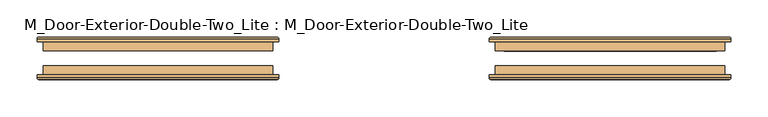
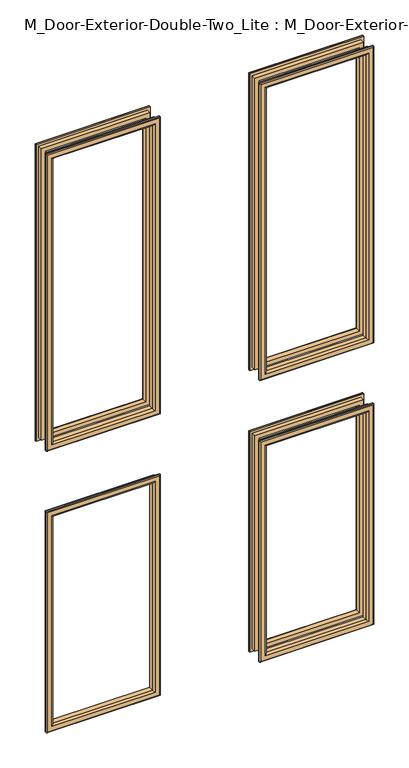
"""IFC4 building model written with IfcOpenShell, lengths in millimetres: door geometry, M_Door-Exterior-Double-Two_Lite : M_Door-Exterior-Double-Two_Lite."""

from ifc_helpers import new_model, si_unit, frame, origin, place, context, project, spatial, ellipse_curve, source, transform, mapped, element, save
from ifc_brep_helpers import plane_surface, cylinder_surface, advanced_brep


def m_door_exterior_double_two_lite_m_door_exterior_double_two_3ba58653(model_context):
    return source(origin(), model_context, "Body", "AdvancedBrep", [
        advanced_brep(
        [(-459.6, 63.15, 1100.0), (-459.6, 50.65, 1100.0), (-459.6, 50.65, 1980.0), (-459.6, 63.15, 1980.0), (-447.6, 49.65, 1112.0), (-447.6, 63.15, 1112.0), (-447.6, 63.15, 1968.0), (-447.6, 49.65, 1968.0), (-452.6, 44.65, 1107.0), (-452.6, 44.65, 1973.0), (-467.6, 46.65, 1092.0), (-465.6, 44.65, 1094.0), (-465.6, 44.65, 1986.0), (-467.6, 46.65, 1988.0), (-467.6, 50.65, 1092.0), (-467.6, 50.65, 1988.0), (-150.0, 50.65, 1980.0), (-150.0, 63.15, 1980.0), (-162.0, 63.15, 1968.0), (-162.0, 49.65, 1968.0), (-157.0, 44.65, 1973.0), (-144.0, 44.65, 1986.0), (-142.0, 46.65, 1988.0), (-142.0, 50.65, 1988.0), (-150.0, 50.65, 1100.0), (-150.0, 63.15, 1100.0), (-162.0, 63.15, 1112.0), (-162.0, 49.65, 1112.0), (-157.0, 44.65, 1107.0), (-144.0, 44.65, 1094.0), (-142.0, 46.65, 1092.0), (-142.0, 50.65, 1092.0)],
        [
            (0, 1),
            (1, 2),
            (2, 3),
            (3, 0),
            (4, 5),
            (5, 6),
            (6, 7),
            (7, 4),
            (8, 4, ellipse_curve(frame((-452.6, 49.65, 1107.0), z_axis=(-0.7071067811865475, 0.0, 0.7071067811865475), x_axis=(-0.7071067811865474, 0.0, -0.7071067811865476)), 7.0710678, 5.0)),
            (7, 9, ellipse_curve(frame((-452.6, 49.65, 1973.0), z_axis=(-0.7071067811865475, 0.0, -0.7071067811865475), x_axis=(0.7071067811865474, 0.0, -0.7071067811865476)), 7.0710678, 5.0)),
            (9, 8),
            (10, 11, ellipse_curve(frame((-465.6, 46.65, 1094.0), z_axis=(-0.7071067811865475, 0.0, 0.7071067811865475), x_axis=(-0.7071067811865474, 0.0, -0.7071067811865476)), 2.8284271, 2.0)),
            (11, 12),
            (12, 13, ellipse_curve(frame((-465.6, 46.65, 1986.0), z_axis=(-0.7071067811865475, 0.0, -0.7071067811865475), x_axis=(0.7071067811865474, 0.0, -0.7071067811865476)), 2.8284271, 2.0)),
            (13, 10),
            (14, 10),
            (13, 15),
            (15, 14),
            (2, 16),
            (16, 17),
            (17, 3),
            (6, 18),
            (18, 19),
            (19, 7),
            (19, 20, ellipse_curve(frame((-157.0, 49.65, 1973.0), z_axis=(-0.7071067811865475, 0.0, 0.7071067811865475), x_axis=(-0.7071067811865476, 0.0, -0.7071067811865474)), 7.0710678, 5.0)),
            (20, 9),
            (12, 21),
            (21, 22, ellipse_curve(frame((-144.0, 46.65, 1986.0), z_axis=(-0.7071067811865475, 0.0, 0.7071067811865475), x_axis=(-0.7071067811865476, 0.0, -0.7071067811865474)), 2.8284271, 2.0)),
            (22, 13),
            (22, 23),
            (23, 15),
            (16, 24),
            (24, 25),
            (25, 17),
            (18, 26),
            (26, 27),
            (27, 19),
            (27, 28, ellipse_curve(frame((-157.0, 49.65, 1107.0), z_axis=(0.7071067811865475, 0.0, 0.7071067811865475), x_axis=(-0.7071067811865474, 0.0, 0.7071067811865476)), 7.0710678, 5.0)),
            (28, 20),
            (21, 29),
            (29, 30, ellipse_curve(frame((-144.0, 46.65, 1094.0), z_axis=(0.7071067811865475, 0.0, 0.7071067811865475), x_axis=(-0.7071067811865474, 0.0, 0.7071067811865476)), 2.8284271, 2.0)),
            (30, 22),
            (30, 31),
            (31, 23),
            (31, 14),
            (1, 24),
            (0, 25),
            (5, 26),
            (4, 27),
            (8, 28),
            (11, 29),
            (10, 30),
        ],
        [
            plane_surface(frame((-459.6, 50.65, 1100.0), z_axis=(-1.0, 0.0, 0.0), x_axis=(0.0, 0.0, 1.0))),
            plane_surface(frame((-447.6, 63.15, 1112.0), z_axis=(1.0, 0.0, 0.0), x_axis=(0.0, 0.0, 1.0))),
            cylinder_surface(frame((-452.6, 49.65, 1100.0), z_axis=(0.0, 0.0, -1.0), x_axis=(-1.0, 0.0, 0.0)), 5.0),
            cylinder_surface(frame((-465.6, 46.65, 1100.0), z_axis=(0.0, 0.0, -1.0), x_axis=(-1.0, 0.0, 0.0)), 2.0),
            plane_surface(frame((-467.6, 46.65, 1092.0), z_axis=(-1.0, 0.0, 0.0), x_axis=(0.0, 0.0, 1.0))),
            plane_surface(frame((-459.6, 50.65, 1980.0), z_axis=(0.0, 0.0, 1.0), x_axis=(1.0, 0.0, 0.0))),
            plane_surface(frame((-447.6, 63.15, 1968.0), z_axis=(0.0, 0.0, -1.0), x_axis=(1.0, 0.0, 0.0))),
            cylinder_surface(frame((-459.6, 49.65, 1973.0), z_axis=(-1.0, 0.0, 0.0), x_axis=(0.0, 0.0, 1.0)), 5.0),
            cylinder_surface(frame((-459.6, 46.65, 1986.0), z_axis=(-1.0, 0.0, 0.0), x_axis=(0.0, 0.0, 1.0)), 2.0),
            plane_surface(frame((-467.6, 46.65, 1988.0), z_axis=(0.0, 0.0, 1.0), x_axis=(1.0, 0.0, 0.0))),
            plane_surface(frame((-150.0, 50.65, 1980.0), z_axis=(1.0, 0.0, 0.0), x_axis=(0.0, 0.0, -1.0))),
            plane_surface(frame((-162.0, 63.15, 1968.0), z_axis=(-1.0, 0.0, 0.0), x_axis=(0.0, 0.0, -1.0))),
            cylinder_surface(frame((-157.0, 49.65, 1980.0), z_axis=(0.0, 0.0, 1.0), x_axis=(1.0, 0.0, 0.0)), 5.0),
            cylinder_surface(frame((-144.0, 46.65, 1980.0), z_axis=(0.0, 0.0, 1.0), x_axis=(1.0, 0.0, 0.0)), 2.0),
            plane_surface(frame((-142.0, 46.65, 1988.0), z_axis=(1.0, 0.0, 0.0), x_axis=(0.0, 0.0, -1.0))),
            plane_surface(frame((-142.0, 50.65, 1092.0), z_axis=(0.0, 1.0, 0.0), x_axis=(-1.0, 0.0, 0.0))),
            plane_surface(frame((-150.0, 50.65, 1100.0), z_axis=(0.0, 0.0, -1.0), x_axis=(-1.0, 0.0, 0.0))),
            plane_surface(frame((-150.0, 63.15, 1100.0), z_axis=(0.0, 1.0, 0.0), x_axis=(-1.0, 0.0, 0.0))),
            plane_surface(frame((-162.0, 63.15, 1112.0), z_axis=(0.0, 0.0, 1.0), x_axis=(-1.0, 0.0, 0.0))),
            cylinder_surface(frame((-150.0, 49.65, 1107.0), z_axis=(1.0, 0.0, 0.0), x_axis=(0.0, 0.0, -1.0)), 5.0),
            plane_surface(frame((-157.0, 44.65, 1107.0), z_axis=(0.0, -1.0, 0.0), x_axis=(-1.0, 0.0, 0.0))),
            cylinder_surface(frame((-150.0, 46.65, 1094.0), z_axis=(1.0, 0.0, 0.0), x_axis=(0.0, 0.0, -1.0)), 2.0),
            plane_surface(frame((-142.0, 46.65, 1092.0), z_axis=(0.0, 0.0, -1.0), x_axis=(-1.0, 0.0, 0.0))),
        ],
        [
            (0, [[1, 2, 3, 4]]),
            (1, [[5, 6, 7, 8]]),
            (2, [[9, -8, 10, 11]]),
            (3, [[12, 13, 14, 15]]),
            (4, [[16, -15, 17, 18]]),
            (5, [[-3, 19, 20, 21]]),
            (6, [[-7, 22, 23, 24]]),
            (7, [[-10, -24, 25, 26]]),
            (8, [[-14, 27, 28, 29]]),
            (9, [[-17, -29, 30, 31]]),
            (10, [[-20, 32, 33, 34]]),
            (11, [[-23, 35, 36, 37]]),
            (12, [[-25, -37, 38, 39]]),
            (13, [[-28, 40, 41, 42]]),
            (14, [[-30, -42, 43, 44]]),
            (15, [[-31, -44, 45, -18], [46, -32, -19, -2]]),
            (16, [[-33, -46, -1, 47]]),
            (17, [[-21, -34, -47, -4], [48, -35, -22, -6]]),
            (18, [[-36, -48, -5, 49]]),
            (19, [[-38, -49, -9, 50]]),
            (20, [[51, -40, -27, -13], [-26, -39, -50, -11]]),
            (21, [[-41, -51, -12, 52]]),
            (22, [[-43, -52, -16, -45]]),
        ],
    ),
        advanced_brep(
        [(150.0, 63.15, 1100.0), (150.0, 50.65, 1100.0), (150.0, 50.65, 1980.0), (150.0, 63.15, 1980.0), (162.0, 49.65, 1112.0), (162.0, 63.15, 1112.0), (162.0, 63.15, 1968.0), (162.0, 49.65, 1968.0), (157.0, 44.65, 1107.0), (157.0, 44.65, 1973.0), (142.0, 46.65, 1092.0), (144.0, 44.65, 1094.0), (144.0, 44.65, 1986.0), (142.0, 46.65, 1988.0), (142.0, 50.65, 1092.0), (142.0, 50.65, 1988.0), (459.6, 50.65, 1980.0), (459.6, 63.15, 1980.0), (447.6, 63.15, 1968.0), (447.6, 49.65, 1968.0), (452.6, 44.65, 1973.0), (465.6, 44.65, 1986.0), (467.6, 46.65, 1988.0), (467.6, 50.65, 1988.0), (459.6, 50.65, 1100.0), (459.6, 63.15, 1100.0), (447.6, 63.15, 1112.0), (447.6, 49.65, 1112.0), (452.6, 44.65, 1107.0), (465.6, 44.65, 1094.0), (467.6, 46.65, 1092.0), (467.6, 50.65, 1092.0)],
        [
            (0, 1),
            (1, 2),
            (2, 3),
            (3, 0),
            (4, 5),
            (5, 6),
            (6, 7),
            (7, 4),
            (8, 4, ellipse_curve(frame((157.0, 49.65, 1107.0), z_axis=(-0.7071067811865475, 0.0, 0.7071067811865475), x_axis=(-0.7071067811865474, 0.0, -0.7071067811865476)), 7.0710678, 5.0)),
            (7, 9, ellipse_curve(frame((157.0, 49.65, 1973.0), z_axis=(-0.7071067811865475, 0.0, -0.7071067811865475), x_axis=(0.7071067811865474, 0.0, -0.7071067811865476)), 7.0710678, 5.0)),
            (9, 8),
            (10, 11, ellipse_curve(frame((144.0, 46.65, 1094.0), z_axis=(-0.7071067811865475, 0.0, 0.7071067811865475), x_axis=(-0.7071067811865474, 0.0, -0.7071067811865476)), 2.8284271, 2.0)),
            (11, 12),
            (12, 13, ellipse_curve(frame((144.0, 46.65, 1986.0), z_axis=(-0.7071067811865475, 0.0, -0.7071067811865475), x_axis=(0.7071067811865474, 0.0, -0.7071067811865476)), 2.8284271, 2.0)),
            (13, 10),
            (14, 10),
            (13, 15),
            (15, 14),
            (2, 16),
            (16, 17),
            (17, 3),
            (6, 18),
            (18, 19),
            (19, 7),
            (19, 20, ellipse_curve(frame((452.6, 49.65, 1973.0), z_axis=(-0.7071067811865475, 0.0, 0.7071067811865475), x_axis=(-0.7071067811865476, 0.0, -0.7071067811865474)), 7.0710678, 5.0)),
            (20, 9),
            (12, 21),
            (21, 22, ellipse_curve(frame((465.6, 46.65, 1986.0), z_axis=(-0.7071067811865475, 0.0, 0.7071067811865475), x_axis=(-0.7071067811865476, 0.0, -0.7071067811865474)), 2.8284271, 2.0)),
            (22, 13),
            (22, 23),
            (23, 15),
            (16, 24),
            (24, 25),
            (25, 17),
            (18, 26),
            (26, 27),
            (27, 19),
            (27, 28, ellipse_curve(frame((452.6, 49.65, 1107.0), z_axis=(0.7071067811865475, 0.0, 0.7071067811865475), x_axis=(-0.7071067811865474, 0.0, 0.7071067811865476)), 7.0710678, 5.0)),
            (28, 20),
            (21, 29),
            (29, 30, ellipse_curve(frame((465.6, 46.65, 1094.0), z_axis=(0.7071067811865475, 0.0, 0.7071067811865475), x_axis=(-0.7071067811865474, 0.0, 0.7071067811865476)), 2.8284271, 2.0)),
            (30, 22),
            (30, 31),
            (31, 23),
            (31, 14),
            (1, 24),
            (0, 25),
            (5, 26),
            (4, 27),
            (8, 28),
            (11, 29),
            (10, 30),
        ],
        [
            plane_surface(frame((150.0, 50.65, 1100.0), z_axis=(-1.0, 0.0, 0.0), x_axis=(0.0, 0.0, 1.0))),
            plane_surface(frame((162.0, 63.15, 1112.0), z_axis=(1.0, 0.0, 0.0), x_axis=(0.0, 0.0, 1.0))),
            cylinder_surface(frame((157.0, 49.65, 1100.0), z_axis=(0.0, 0.0, -1.0), x_axis=(-1.0, 0.0, 0.0)), 5.0),
            cylinder_surface(frame((144.0, 46.65, 1100.0), z_axis=(0.0, 0.0, -1.0), x_axis=(-1.0, 0.0, 0.0)), 2.0),
            plane_surface(frame((142.0, 46.65, 1092.0), z_axis=(-1.0, 0.0, 0.0), x_axis=(0.0, 0.0, 1.0))),
            plane_surface(frame((150.0, 50.65, 1980.0), z_axis=(0.0, 0.0, 1.0), x_axis=(1.0, 0.0, 0.0))),
            plane_surface(frame((162.0, 63.15, 1968.0), z_axis=(0.0, 0.0, -1.0), x_axis=(1.0, 0.0, 0.0))),
            cylinder_surface(frame((150.0, 49.65, 1973.0), z_axis=(-1.0, 0.0, 0.0), x_axis=(0.0, 0.0, 1.0)), 5.0),
            cylinder_surface(frame((150.0, 46.65, 1986.0), z_axis=(-1.0, 0.0, 0.0), x_axis=(0.0, 0.0, 1.0)), 2.0),
            plane_surface(frame((142.0, 46.65, 1988.0), z_axis=(0.0, 0.0, 1.0), x_axis=(1.0, 0.0, 0.0))),
            plane_surface(frame((459.6, 50.65, 1980.0), z_axis=(1.0, 0.0, 0.0), x_axis=(0.0, 0.0, -1.0))),
            plane_surface(frame((447.6, 63.15, 1968.0), z_axis=(-1.0, 0.0, 0.0), x_axis=(0.0, 0.0, -1.0))),
            cylinder_surface(frame((452.6, 49.65, 1980.0), z_axis=(0.0, 0.0, 1.0), x_axis=(1.0, 0.0, 0.0)), 5.0),
            cylinder_surface(frame((465.6, 46.65, 1980.0), z_axis=(0.0, 0.0, 1.0), x_axis=(1.0, 0.0, 0.0)), 2.0),
            plane_surface(frame((467.6, 46.65, 1988.0), z_axis=(1.0, 0.0, 0.0), x_axis=(0.0, 0.0, -1.0))),
            plane_surface(frame((467.6, 50.65, 1092.0), z_axis=(0.0, 1.0, 0.0), x_axis=(-1.0, 0.0, 0.0))),
            plane_surface(frame((459.6, 50.65, 1100.0), z_axis=(0.0, 0.0, -1.0), x_axis=(-1.0, 0.0, 0.0))),
            plane_surface(frame((459.6, 63.15, 1100.0), z_axis=(0.0, 1.0, 0.0), x_axis=(-1.0, 0.0, 0.0))),
            plane_surface(frame((447.6, 63.15, 1112.0), z_axis=(0.0, 0.0, 1.0), x_axis=(-1.0, 0.0, 0.0))),
            cylinder_surface(frame((459.6, 49.65, 1107.0), z_axis=(1.0, 0.0, 0.0), x_axis=(0.0, 0.0, -1.0)), 5.0),
            plane_surface(frame((452.6, 44.65, 1107.0), z_axis=(0.0, -1.0, 0.0), x_axis=(-1.0, 0.0, 0.0))),
            cylinder_surface(frame((459.6, 46.65, 1094.0), z_axis=(1.0, 0.0, 0.0), x_axis=(0.0, 0.0, -1.0)), 2.0),
            plane_surface(frame((467.6, 46.65, 1092.0), z_axis=(0.0, 0.0, -1.0), x_axis=(-1.0, 0.0, 0.0))),
        ],
        [
            (0, [[1, 2, 3, 4]]),
            (1, [[5, 6, 7, 8]]),
            (2, [[9, -8, 10, 11]]),
            (3, [[12, 13, 14, 15]]),
            (4, [[16, -15, 17, 18]]),
            (5, [[-3, 19, 20, 21]]),
            (6, [[-7, 22, 23, 24]]),
            (7, [[-10, -24, 25, 26]]),
            (8, [[-14, 27, 28, 29]]),
            (9, [[-17, -29, 30, 31]]),
            (10, [[-20, 32, 33, 34]]),
            (11, [[-23, 35, 36, 37]]),
            (12, [[-25, -37, 38, 39]]),
            (13, [[-28, 40, 41, 42]]),
            (14, [[-30, -42, 43, 44]]),
            (15, [[-31, -44, 45, -18], [46, -32, -19, -2]]),
            (16, [[-33, -46, -1, 47]]),
            (17, [[-21, -34, -47, -4], [48, -35, -22, -6]]),
            (18, [[-36, -48, -5, 49]]),
            (19, [[-38, -49, -9, 50]]),
            (20, [[51, -40, -27, -13], [-26, -39, -50, -11]]),
            (21, [[-41, -51, -12, 52]]),
            (22, [[-43, -52, -16, -45]]),
        ],
    ),
        advanced_brep(
        [(150.0, 63.15, 250.0), (150.0, 50.65, 250.0), (150.0, 50.65, 900.0), (150.0, 63.15, 900.0), (162.0, 49.65, 262.0), (162.0, 63.15, 262.0), (162.0, 63.15, 888.0), (162.0, 49.65, 888.0), (157.0, 44.65, 257.0), (157.0, 44.65, 893.0), (142.0, 46.65, 242.0), (144.0, 44.65, 244.0), (144.0, 44.65, 906.0), (142.0, 46.65, 908.0), (142.0, 50.65, 242.0), (142.0, 50.65, 908.0), (459.6, 50.65, 900.0), (459.6, 63.15, 900.0), (447.6, 63.15, 888.0), (447.6, 49.65, 888.0), (452.6, 44.65, 893.0), (465.6, 44.65, 906.0), (467.6, 46.65, 908.0), (467.6, 50.65, 908.0), (459.6, 50.65, 250.0), (459.6, 63.15, 250.0), (447.6, 63.15, 262.0), (447.6, 49.65, 262.0), (452.6, 44.65, 257.0), (465.6, 44.65, 244.0), (467.6, 46.65, 242.0), (467.6, 50.65, 242.0)],
        [
            (0, 1),
            (1, 2),
            (2, 3),
            (3, 0),
            (4, 5),
            (5, 6),
            (6, 7),
            (7, 4),
            (8, 4, ellipse_curve(frame((157.0, 49.65, 257.0), z_axis=(-0.7071067811865475, 0.0, 0.7071067811865475), x_axis=(-0.7071067811865474, 0.0, -0.7071067811865476)), 7.0710678, 5.0)),
            (7, 9, ellipse_curve(frame((157.0, 49.65, 893.0), z_axis=(-0.7071067811865475, 0.0, -0.7071067811865475), x_axis=(0.7071067811865474, 0.0, -0.7071067811865476)), 7.0710678, 5.0)),
            (9, 8),
            (10, 11, ellipse_curve(frame((144.0, 46.65, 244.0), z_axis=(-0.7071067811865475, 0.0, 0.7071067811865475), x_axis=(-0.7071067811865474, 0.0, -0.7071067811865476)), 2.8284271, 2.0)),
            (11, 12),
            (12, 13, ellipse_curve(frame((144.0, 46.65, 906.0), z_axis=(-0.7071067811865475, 0.0, -0.7071067811865475), x_axis=(0.7071067811865474, 0.0, -0.7071067811865476)), 2.8284271, 2.0)),
            (13, 10),
            (14, 10),
            (13, 15),
            (15, 14),
            (2, 16),
            (16, 17),
            (17, 3),
            (6, 18),
            (18, 19),
            (19, 7),
            (19, 20, ellipse_curve(frame((452.6, 49.65, 893.0), z_axis=(-0.7071067811865475, 0.0, 0.7071067811865475), x_axis=(-0.7071067811865476, 0.0, -0.7071067811865474)), 7.0710678, 5.0)),
            (20, 9),
            (12, 21),
            (21, 22, ellipse_curve(frame((465.6, 46.65, 906.0), z_axis=(-0.7071067811865475, 0.0, 0.7071067811865475), x_axis=(-0.7071067811865476, 0.0, -0.7071067811865474)), 2.8284271, 2.0)),
            (22, 13),
            (22, 23),
            (23, 15),
            (16, 24),
            (24, 25),
            (25, 17),
            (18, 26),
            (26, 27),
            (27, 19),
            (27, 28, ellipse_curve(frame((452.6, 49.65, 257.0), z_axis=(0.7071067811865475, 0.0, 0.7071067811865475), x_axis=(-0.7071067811865474, 0.0, 0.7071067811865476)), 7.0710678, 5.0)),
            (28, 20),
            (21, 29),
            (29, 30, ellipse_curve(frame((465.6, 46.65, 244.0), z_axis=(0.7071067811865475, 0.0, 0.7071067811865475), x_axis=(-0.7071067811865474, 0.0, 0.7071067811865476)), 2.8284271, 2.0)),
            (30, 22),
            (30, 31),
            (31, 23),
            (31, 14),
            (1, 24),
            (0, 25),
            (5, 26),
            (4, 27),
            (8, 28),
            (11, 29),
            (10, 30),
        ],
        [
            plane_surface(frame((150.0, 50.65, 250.0), z_axis=(-1.0, 0.0, 0.0), x_axis=(0.0, 0.0, 1.0))),
            plane_surface(frame((162.0, 63.15, 262.0), z_axis=(1.0, 0.0, 0.0), x_axis=(0.0, 0.0, 1.0))),
            cylinder_surface(frame((157.0, 49.65, 250.0), z_axis=(0.0, 0.0, -1.0), x_axis=(-1.0, 0.0, 0.0)), 5.0),
            cylinder_surface(frame((144.0, 46.65, 250.0), z_axis=(0.0, 0.0, -1.0), x_axis=(-1.0, 0.0, 0.0)), 2.0),
            plane_surface(frame((142.0, 46.65, 242.0), z_axis=(-1.0, 0.0, 0.0), x_axis=(0.0, 0.0, 1.0))),
            plane_surface(frame((150.0, 50.65, 900.0), z_axis=(0.0, 0.0, 1.0), x_axis=(1.0, 0.0, 0.0))),
            plane_surface(frame((162.0, 63.15, 888.0), z_axis=(0.0, 0.0, -1.0), x_axis=(1.0, 0.0, 0.0))),
            cylinder_surface(frame((150.0, 49.65, 893.0), z_axis=(-1.0, 0.0, 0.0), x_axis=(0.0, 0.0, 1.0)), 5.0),
            cylinder_surface(frame((150.0, 46.65, 906.0), z_axis=(-1.0, 0.0, 0.0), x_axis=(0.0, 0.0, 1.0)), 2.0),
            plane_surface(frame((142.0, 46.65, 908.0), z_axis=(0.0, 0.0, 1.0), x_axis=(1.0, 0.0, 0.0))),
            plane_surface(frame((459.6, 50.65, 900.0), z_axis=(1.0, 0.0, 0.0), x_axis=(0.0, 0.0, -1.0))),
            plane_surface(frame((447.6, 63.15, 888.0), z_axis=(-1.0, 0.0, 0.0), x_axis=(0.0, 0.0, -1.0))),
            cylinder_surface(frame((452.6, 49.65, 900.0), z_axis=(0.0, 0.0, 1.0), x_axis=(1.0, 0.0, 0.0)), 5.0),
            cylinder_surface(frame((465.6, 46.65, 900.0), z_axis=(0.0, 0.0, 1.0), x_axis=(1.0, 0.0, 0.0)), 2.0),
            plane_surface(frame((467.6, 46.65, 908.0), z_axis=(1.0, 0.0, 0.0), x_axis=(0.0, 0.0, -1.0))),
            plane_surface(frame((467.6, 50.65, 242.0), z_axis=(0.0, 1.0, 0.0), x_axis=(-1.0, 0.0, 0.0))),
            plane_surface(frame((459.6, 50.65, 250.0), z_axis=(0.0, 0.0, -1.0), x_axis=(-1.0, 0.0, 0.0))),
            plane_surface(frame((459.6, 63.15, 250.0), z_axis=(0.0, 1.0, 0.0), x_axis=(-1.0, 0.0, 0.0))),
            plane_surface(frame((447.6, 63.15, 262.0), z_axis=(0.0, 0.0, 1.0), x_axis=(-1.0, 0.0, 0.0))),
            cylinder_surface(frame((459.6, 49.65, 257.0), z_axis=(1.0, 0.0, 0.0), x_axis=(0.0, 0.0, -1.0)), 5.0),
            plane_surface(frame((452.6, 44.65, 257.0), z_axis=(0.0, -1.0, 0.0), x_axis=(-1.0, 0.0, 0.0))),
            cylinder_surface(frame((459.6, 46.65, 244.0), z_axis=(1.0, 0.0, 0.0), x_axis=(0.0, 0.0, -1.0)), 2.0),
            plane_surface(frame((467.6, 46.65, 242.0), z_axis=(0.0, 0.0, -1.0), x_axis=(-1.0, 0.0, 0.0))),
        ],
        [
            (0, [[1, 2, 3, 4]]),
            (1, [[5, 6, 7, 8]]),
            (2, [[9, -8, 10, 11]]),
            (3, [[12, 13, 14, 15]]),
            (4, [[16, -15, 17, 18]]),
            (5, [[-3, 19, 20, 21]]),
            (6, [[-7, 22, 23, 24]]),
            (7, [[-10, -24, 25, 26]]),
            (8, [[-14, 27, 28, 29]]),
            (9, [[-17, -29, 30, 31]]),
            (10, [[-20, 32, 33, 34]]),
            (11, [[-23, 35, 36, 37]]),
            (12, [[-25, -37, 38, 39]]),
            (13, [[-28, 40, 41, 42]]),
            (14, [[-30, -42, 43, 44]]),
            (15, [[-31, -44, 45, -18], [46, -32, -19, -2]]),
            (16, [[-33, -46, -1, 47]]),
            (17, [[-21, -34, -47, -4], [48, -35, -22, -6]]),
            (18, [[-36, -48, -5, 49]]),
            (19, [[-38, -49, -9, 50]]),
            (20, [[51, -40, -27, -13], [-26, -39, -50, -11]]),
            (21, [[-41, -51, -12, 52]]),
            (22, [[-43, -52, -16, -45]]),
        ],
    ),
        advanced_brep(
        [(-459.6, 63.15, 250.0), (-459.6, 50.65, 250.0), (-459.6, 50.65, 900.0), (-459.6, 63.15, 900.0), (-447.6, 49.65, 262.0), (-447.6, 63.15, 262.0), (-447.6, 63.15, 888.0), (-447.6, 49.65, 888.0), (-452.6, 44.65, 257.0), (-452.6, 44.65, 893.0), (-467.6, 46.65, 242.0), (-465.6, 44.65, 244.0), (-465.6, 44.65, 906.0), (-467.6, 46.65, 908.0), (-467.6, 50.65, 242.0), (-467.6, 50.65, 908.0), (-150.0, 50.65, 900.0), (-150.0, 63.15, 900.0), (-162.0, 63.15, 888.0), (-162.0, 49.65, 888.0), (-157.0, 44.65, 893.0), (-144.0, 44.65, 906.0), (-142.0, 46.65, 908.0), (-142.0, 50.65, 908.0), (-150.0, 50.65, 250.0), (-150.0, 63.15, 250.0), (-162.0, 63.15, 262.0), (-162.0, 49.65, 262.0), (-157.0, 44.65, 257.0), (-144.0, 44.65, 244.0), (-142.0, 46.65, 242.0), (-142.0, 50.65, 242.0)],
        [
            (0, 1),
            (1, 2),
            (2, 3),
            (3, 0),
            (4, 5),
            (5, 6),
            (6, 7),
            (7, 4),
            (8, 4, ellipse_curve(frame((-452.6, 49.65, 257.0), z_axis=(-0.7071067811865475, 0.0, 0.7071067811865475), x_axis=(-0.7071067811865474, 0.0, -0.7071067811865476)), 7.0710678, 5.0)),
            (7, 9, ellipse_curve(frame((-452.6, 49.65, 893.0), z_axis=(-0.7071067811865475, 0.0, -0.7071067811865475), x_axis=(0.7071067811865474, 0.0, -0.7071067811865476)), 7.0710678, 5.0)),
            (9, 8),
            (10, 11, ellipse_curve(frame((-465.6, 46.65, 244.0), z_axis=(-0.7071067811865475, 0.0, 0.7071067811865475), x_axis=(-0.7071067811865474, 0.0, -0.7071067811865476)), 2.8284271, 2.0)),
            (11, 12),
            (12, 13, ellipse_curve(frame((-465.6, 46.65, 906.0), z_axis=(-0.7071067811865475, 0.0, -0.7071067811865475), x_axis=(0.7071067811865474, 0.0, -0.7071067811865476)), 2.8284271, 2.0)),
            (13, 10),
            (14, 10),
            (13, 15),
            (15, 14),
            (2, 16),
            (16, 17),
            (17, 3),
            (6, 18),
            (18, 19),
            (19, 7),
            (19, 20, ellipse_curve(frame((-157.0, 49.65, 893.0), z_axis=(-0.7071067811865475, 0.0, 0.7071067811865475), x_axis=(-0.7071067811865476, 0.0, -0.7071067811865474)), 7.0710678, 5.0)),
            (20, 9),
            (12, 21),
            (21, 22, ellipse_curve(frame((-144.0, 46.65, 906.0), z_axis=(-0.7071067811865475, 0.0, 0.7071067811865475), x_axis=(-0.7071067811865476, 0.0, -0.7071067811865474)), 2.8284271, 2.0)),
            (22, 13),
            (22, 23),
            (23, 15),
            (16, 24),
            (24, 25),
            (25, 17),
            (18, 26),
            (26, 27),
            (27, 19),
            (27, 28, ellipse_curve(frame((-157.0, 49.65, 257.0), z_axis=(0.7071067811865475, 0.0, 0.7071067811865475), x_axis=(-0.7071067811865474, 0.0, 0.7071067811865476)), 7.0710678, 5.0)),
            (28, 20),
            (21, 29),
            (29, 30, ellipse_curve(frame((-144.0, 46.65, 244.0), z_axis=(0.7071067811865475, 0.0, 0.7071067811865475), x_axis=(-0.7071067811865474, 0.0, 0.7071067811865476)), 2.8284271, 2.0)),
            (30, 22),
            (30, 31),
            (31, 23),
            (31, 14),
            (1, 24),
            (0, 25),
            (5, 26),
            (4, 27),
            (8, 28),
            (11, 29),
            (10, 30),
        ],
        [
            plane_surface(frame((-459.6, 50.65, 250.0), z_axis=(-1.0, 0.0, 0.0), x_axis=(0.0, 0.0, 1.0))),
            plane_surface(frame((-447.6, 63.15, 262.0), z_axis=(1.0, 0.0, 0.0), x_axis=(0.0, 0.0, 1.0))),
            cylinder_surface(frame((-452.6, 49.65, 250.0), z_axis=(0.0, 0.0, -1.0), x_axis=(-1.0, 0.0, 0.0)), 5.0),
            cylinder_surface(frame((-465.6, 46.65, 250.0), z_axis=(0.0, 0.0, -1.0), x_axis=(-1.0, 0.0, 0.0)), 2.0),
            plane_surface(frame((-467.6, 46.65, 242.0), z_axis=(-1.0, 0.0, 0.0), x_axis=(0.0, 0.0, 1.0))),
            plane_surface(frame((-459.6, 50.65, 900.0), z_axis=(0.0, 0.0, 1.0), x_axis=(1.0, 0.0, 0.0))),
            plane_surface(frame((-447.6, 63.15, 888.0), z_axis=(0.0, 0.0, -1.0), x_axis=(1.0, 0.0, 0.0))),
            cylinder_surface(frame((-459.6, 49.65, 893.0), z_axis=(-1.0, 0.0, 0.0), x_axis=(0.0, 0.0, 1.0)), 5.0),
            cylinder_surface(frame((-459.6, 46.65, 906.0), z_axis=(-1.0, 0.0, 0.0), x_axis=(0.0, 0.0, 1.0)), 2.0),
            plane_surface(frame((-467.6, 46.65, 908.0), z_axis=(0.0, 0.0, 1.0), x_axis=(1.0, 0.0, 0.0))),
            plane_surface(frame((-150.0, 50.65, 900.0), z_axis=(1.0, 0.0, 0.0), x_axis=(0.0, 0.0, -1.0))),
            plane_surface(frame((-162.0, 63.15, 888.0), z_axis=(-1.0, 0.0, 0.0), x_axis=(0.0, 0.0, -1.0))),
            cylinder_surface(frame((-157.0, 49.65, 900.0), z_axis=(0.0, 0.0, 1.0), x_axis=(1.0, 0.0, 0.0)), 5.0),
            cylinder_surface(frame((-144.0, 46.65, 900.0), z_axis=(0.0, 0.0, 1.0), x_axis=(1.0, 0.0, 0.0)), 2.0),
            plane_surface(frame((-142.0, 46.65, 908.0), z_axis=(1.0, 0.0, 0.0), x_axis=(0.0, 0.0, -1.0))),
            plane_surface(frame((-142.0, 50.65, 242.0), z_axis=(0.0, 1.0, 0.0), x_axis=(-1.0, 0.0, 0.0))),
            plane_surface(frame((-150.0, 50.65, 250.0), z_axis=(0.0, 0.0, -1.0), x_axis=(-1.0, 0.0, 0.0))),
            plane_surface(frame((-150.0, 63.15, 250.0), z_axis=(0.0, 1.0, 0.0), x_axis=(-1.0, 0.0, 0.0))),
            plane_surface(frame((-162.0, 63.15, 262.0), z_axis=(0.0, 0.0, 1.0), x_axis=(-1.0, 0.0, 0.0))),
            cylinder_surface(frame((-150.0, 49.65, 257.0), z_axis=(1.0, 0.0, 0.0), x_axis=(0.0, 0.0, -1.0)), 5.0),
            plane_surface(frame((-157.0, 44.65, 257.0), z_axis=(0.0, -1.0, 0.0), x_axis=(-1.0, 0.0, 0.0))),
            cylinder_surface(frame((-150.0, 46.65, 244.0), z_axis=(1.0, 0.0, 0.0), x_axis=(0.0, 0.0, -1.0)), 2.0),
            plane_surface(frame((-142.0, 46.65, 242.0), z_axis=(0.0, 0.0, -1.0), x_axis=(-1.0, 0.0, 0.0))),
        ],
        [
            (0, [[1, 2, 3, 4]]),
            (1, [[5, 6, 7, 8]]),
            (2, [[9, -8, 10, 11]]),
            (3, [[12, 13, 14, 15]]),
            (4, [[16, -15, 17, 18]]),
            (5, [[-3, 19, 20, 21]]),
            (6, [[-7, 22, 23, 24]]),
            (7, [[-10, -24, 25, 26]]),
            (8, [[-14, 27, 28, 29]]),
            (9, [[-17, -29, 30, 31]]),
            (10, [[-20, 32, 33, 34]]),
            (11, [[-23, 35, 36, 37]]),
            (12, [[-25, -37, 38, 39]]),
            (13, [[-28, 40, 41, 42]]),
            (14, [[-30, -42, 43, 44]]),
            (15, [[-31, -44, 45, -18], [46, -32, -19, -2]]),
            (16, [[-33, -46, -1, 47]]),
            (17, [[-21, -34, -47, -4], [48, -35, -22, -6]]),
            (18, [[-36, -48, -5, 49]]),
            (19, [[-38, -49, -9, 50]]),
            (20, [[51, -40, -27, -13], [-26, -39, -50, -11]]),
            (21, [[-41, -51, -12, 52]]),
            (22, [[-43, -52, -16, -45]]),
        ],
    ),
        advanced_brep(
        [(-459.6, 83.15, 1980.0), (-459.6, 95.65, 1980.0), (-459.6, 95.65, 1100.0), (-459.6, 83.15, 1100.0), (-447.6, 96.65, 1968.0), (-447.6, 83.15, 1968.0), (-447.6, 83.15, 1112.0), (-447.6, 96.65, 1112.0), (-452.6, 101.65, 1973.0), (-452.6, 101.65, 1107.0), (-467.6, 99.65, 1988.0), (-465.6, 101.65, 1986.0), (-465.6, 101.65, 1094.0), (-467.6, 99.65, 1092.0), (-467.6, 95.65, 1988.0), (-467.6, 95.65, 1092.0), (-150.0, 95.65, 1100.0), (-150.0, 83.15, 1100.0), (-162.0, 83.15, 1112.0), (-162.0, 96.65, 1112.0), (-157.0, 101.65, 1107.0), (-144.0, 101.65, 1094.0), (-142.0, 99.65, 1092.0), (-142.0, 95.65, 1092.0), (-150.0, 95.65, 1980.0), (-150.0, 83.15, 1980.0), (-162.0, 83.15, 1968.0), (-162.0, 96.65, 1968.0), (-157.0, 101.65, 1973.0), (-144.0, 101.65, 1986.0), (-142.0, 99.65, 1988.0), (-142.0, 95.65, 1988.0)],
        [
            (0, 1),
            (1, 2),
            (2, 3),
            (3, 0),
            (4, 5),
            (5, 6),
            (6, 7),
            (7, 4),
            (8, 4, ellipse_curve(frame((-452.6, 96.65, 1973.0), z_axis=(-0.7071067811865475, 0.0, -0.7071067811865475), x_axis=(-0.7071067811865474, 0.0, 0.7071067811865476)), 7.0710678, 5.0)),
            (7, 9, ellipse_curve(frame((-452.6, 96.65, 1107.0), z_axis=(-0.7071067811865475, 0.0, 0.7071067811865475), x_axis=(0.7071067811865474, 0.0, 0.7071067811865476)), 7.0710678, 5.0)),
            (9, 8),
            (10, 11, ellipse_curve(frame((-465.6, 99.65, 1986.0), z_axis=(-0.7071067811865475, 0.0, -0.7071067811865475), x_axis=(-0.7071067811865474, 0.0, 0.7071067811865476)), 2.8284271, 2.0)),
            (11, 12),
            (12, 13, ellipse_curve(frame((-465.6, 99.65, 1094.0), z_axis=(-0.7071067811865475, 0.0, 0.7071067811865475), x_axis=(0.7071067811865474, 0.0, 0.7071067811865476)), 2.8284271, 2.0)),
            (13, 10),
            (14, 10),
            (13, 15),
            (15, 14),
            (2, 16),
            (16, 17),
            (17, 3),
            (6, 18),
            (18, 19),
            (19, 7),
            (19, 20, ellipse_curve(frame((-157.0, 96.65, 1107.0), z_axis=(-0.7071067811865475, 0.0, -0.7071067811865475), x_axis=(-0.7071067811865476, 0.0, 0.7071067811865474)), 7.0710678, 5.0)),
            (20, 9),
            (12, 21),
            (21, 22, ellipse_curve(frame((-144.0, 99.65, 1094.0), z_axis=(-0.7071067811865475, 0.0, -0.7071067811865475), x_axis=(-0.7071067811865476, 0.0, 0.7071067811865474)), 2.8284271, 2.0)),
            (22, 13),
            (22, 23),
            (23, 15),
            (16, 24),
            (24, 25),
            (25, 17),
            (18, 26),
            (26, 27),
            (27, 19),
            (27, 28, ellipse_curve(frame((-157.0, 96.65, 1973.0), z_axis=(0.7071067811865475, 0.0, -0.7071067811865475), x_axis=(-0.7071067811865474, 0.0, -0.7071067811865476)), 7.0710678, 5.0)),
            (28, 20),
            (21, 29),
            (29, 30, ellipse_curve(frame((-144.0, 99.65, 1986.0), z_axis=(0.7071067811865475, 0.0, -0.7071067811865475), x_axis=(-0.7071067811865474, 0.0, -0.7071067811865476)), 2.8284271, 2.0)),
            (30, 22),
            (30, 31),
            (31, 23),
            (31, 14),
            (1, 24),
            (0, 25),
            (5, 26),
            (4, 27),
            (8, 28),
            (11, 29),
            (10, 30),
        ],
        [
            plane_surface(frame((-459.6, 95.65, 1980.0), z_axis=(-1.0, 0.0, 0.0), x_axis=(0.0, 0.0, -1.0))),
            plane_surface(frame((-447.6, 83.15, 1968.0), z_axis=(1.0, 0.0, 0.0), x_axis=(0.0, 0.0, -1.0))),
            cylinder_surface(frame((-452.6, 96.65, 1980.0), z_axis=(0.0, 0.0, 1.0), x_axis=(-1.0, 0.0, 0.0)), 5.0),
            cylinder_surface(frame((-465.6, 99.65, 1980.0), z_axis=(0.0, 0.0, 1.0), x_axis=(-1.0, 0.0, 0.0)), 2.0),
            plane_surface(frame((-467.6, 99.65, 1988.0), z_axis=(-1.0, 0.0, 0.0), x_axis=(0.0, 0.0, -1.0))),
            plane_surface(frame((-459.6, 95.65, 1100.0), z_axis=(0.0, 0.0, -1.0), x_axis=(1.0, 0.0, 0.0))),
            plane_surface(frame((-447.6, 83.15, 1112.0), z_axis=(0.0, 0.0, 1.0), x_axis=(1.0, 0.0, 0.0))),
            cylinder_surface(frame((-459.6, 96.65, 1107.0), z_axis=(-1.0, 0.0, 0.0), x_axis=(0.0, 0.0, -1.0)), 5.0),
            cylinder_surface(frame((-459.6, 99.65, 1094.0), z_axis=(-1.0, 0.0, 0.0), x_axis=(0.0, 0.0, -1.0)), 2.0),
            plane_surface(frame((-467.6, 99.65, 1092.0), z_axis=(0.0, 0.0, -1.0), x_axis=(1.0, 0.0, 0.0))),
            plane_surface(frame((-150.0, 95.65, 1100.0), z_axis=(1.0, 0.0, 0.0), x_axis=(0.0, 0.0, 1.0))),
            plane_surface(frame((-162.0, 83.15, 1112.0), z_axis=(-1.0, 0.0, 0.0), x_axis=(0.0, 0.0, 1.0))),
            cylinder_surface(frame((-157.0, 96.65, 1100.0), z_axis=(0.0, 0.0, -1.0), x_axis=(1.0, 0.0, 0.0)), 5.0),
            cylinder_surface(frame((-144.0, 99.65, 1100.0), z_axis=(0.0, 0.0, -1.0), x_axis=(1.0, 0.0, 0.0)), 2.0),
            plane_surface(frame((-142.0, 99.65, 1092.0), z_axis=(1.0, 0.0, 0.0), x_axis=(0.0, 0.0, 1.0))),
            plane_surface(frame((-142.0, 95.65, 1988.0), z_axis=(0.0, -1.0, 0.0), x_axis=(-1.0, 0.0, 0.0))),
            plane_surface(frame((-150.0, 95.65, 1980.0), z_axis=(0.0, 0.0, 1.0), x_axis=(-1.0, 0.0, 0.0))),
            plane_surface(frame((-150.0, 83.15, 1980.0), z_axis=(0.0, -1.0, 0.0), x_axis=(-1.0, 0.0, 0.0))),
            plane_surface(frame((-162.0, 83.15, 1968.0), z_axis=(0.0, 0.0, -1.0), x_axis=(-1.0, 0.0, 0.0))),
            cylinder_surface(frame((-150.0, 96.65, 1973.0), z_axis=(1.0, 0.0, 0.0), x_axis=(0.0, 0.0, 1.0)), 5.0),
            plane_surface(frame((-157.0, 101.65, 1973.0), z_axis=(0.0, 1.0, 0.0), x_axis=(-1.0, 0.0, 0.0))),
            cylinder_surface(frame((-150.0, 99.65, 1986.0), z_axis=(1.0, 0.0, 0.0), x_axis=(0.0, 0.0, 1.0)), 2.0),
            plane_surface(frame((-142.0, 99.65, 1988.0), z_axis=(0.0, 0.0, 1.0), x_axis=(-1.0, 0.0, 0.0))),
        ],
        [
            (0, [[1, 2, 3, 4]]),
            (1, [[5, 6, 7, 8]]),
            (2, [[9, -8, 10, 11]]),
            (3, [[12, 13, 14, 15]]),
            (4, [[16, -15, 17, 18]]),
            (5, [[-3, 19, 20, 21]]),
            (6, [[-7, 22, 23, 24]]),
            (7, [[-10, -24, 25, 26]]),
            (8, [[-14, 27, 28, 29]]),
            (9, [[-17, -29, 30, 31]]),
            (10, [[-20, 32, 33, 34]]),
            (11, [[-23, 35, 36, 37]]),
            (12, [[-25, -37, 38, 39]]),
            (13, [[-28, 40, 41, 42]]),
            (14, [[-30, -42, 43, 44]]),
            (15, [[-31, -44, 45, -18], [46, -32, -19, -2]]),
            (16, [[-33, -46, -1, 47]]),
            (17, [[-21, -34, -47, -4], [48, -35, -22, -6]]),
            (18, [[-36, -48, -5, 49]]),
            (19, [[-38, -49, -9, 50]]),
            (20, [[51, -40, -27, -13], [-26, -39, -50, -11]]),
            (21, [[-41, -51, -12, 52]]),
            (22, [[-43, -52, -16, -45]]),
        ],
    ),
        advanced_brep(
        [(150.0, 83.15, 1980.0), (150.0, 95.65, 1980.0), (150.0, 95.65, 1100.0), (150.0, 83.15, 1100.0), (162.0, 96.65, 1968.0), (162.0, 83.15, 1968.0), (162.0, 83.15, 1112.0), (162.0, 96.65, 1112.0), (157.0, 101.65, 1973.0), (157.0, 101.65, 1107.0), (142.0, 99.65, 1988.0), (144.0, 101.65, 1986.0), (144.0, 101.65, 1094.0), (142.0, 99.65, 1092.0), (142.0, 95.65, 1988.0), (142.0, 95.65, 1092.0), (459.6, 95.65, 1100.0), (459.6, 83.15, 1100.0), (447.6, 83.15, 1112.0), (447.6, 96.65, 1112.0), (452.6, 101.65, 1107.0), (465.6, 101.65, 1094.0), (467.6, 99.65, 1092.0), (467.6, 95.65, 1092.0), (459.6, 95.65, 1980.0), (459.6, 83.15, 1980.0), (447.6, 83.15, 1968.0), (447.6, 96.65, 1968.0), (452.6, 101.65, 1973.0), (465.6, 101.65, 1986.0), (467.6, 99.65, 1988.0), (467.6, 95.65, 1988.0)],
        [
            (0, 1),
            (1, 2),
            (2, 3),
            (3, 0),
            (4, 5),
            (5, 6),
            (6, 7),
            (7, 4),
            (8, 4, ellipse_curve(frame((157.0, 96.65, 1973.0), z_axis=(-0.7071067811865475, 0.0, -0.7071067811865475), x_axis=(-0.7071067811865474, 0.0, 0.7071067811865476)), 7.0710678, 5.0)),
            (7, 9, ellipse_curve(frame((157.0, 96.65, 1107.0), z_axis=(-0.7071067811865475, 0.0, 0.7071067811865475), x_axis=(0.7071067811865474, 0.0, 0.7071067811865476)), 7.0710678, 5.0)),
            (9, 8),
            (10, 11, ellipse_curve(frame((144.0, 99.65, 1986.0), z_axis=(-0.7071067811865475, 0.0, -0.7071067811865475), x_axis=(-0.7071067811865474, 0.0, 0.7071067811865476)), 2.8284271, 2.0)),
            (11, 12),
            (12, 13, ellipse_curve(frame((144.0, 99.65, 1094.0), z_axis=(-0.7071067811865475, 0.0, 0.7071067811865475), x_axis=(0.7071067811865474, 0.0, 0.7071067811865476)), 2.8284271, 2.0)),
            (13, 10),
            (14, 10),
            (13, 15),
            (15, 14),
            (2, 16),
            (16, 17),
            (17, 3),
            (6, 18),
            (18, 19),
            (19, 7),
            (19, 20, ellipse_curve(frame((452.6, 96.65, 1107.0), z_axis=(-0.7071067811865475, 0.0, -0.7071067811865475), x_axis=(-0.7071067811865476, 0.0, 0.7071067811865474)), 7.0710678, 5.0)),
            (20, 9),
            (12, 21),
            (21, 22, ellipse_curve(frame((465.6, 99.65, 1094.0), z_axis=(-0.7071067811865475, 0.0, -0.7071067811865475), x_axis=(-0.7071067811865476, 0.0, 0.7071067811865474)), 2.8284271, 2.0)),
            (22, 13),
            (22, 23),
            (23, 15),
            (16, 24),
            (24, 25),
            (25, 17),
            (18, 26),
            (26, 27),
            (27, 19),
            (27, 28, ellipse_curve(frame((452.6, 96.65, 1973.0), z_axis=(0.7071067811865475, 0.0, -0.7071067811865475), x_axis=(-0.7071067811865474, 0.0, -0.7071067811865476)), 7.0710678, 5.0)),
            (28, 20),
            (21, 29),
            (29, 30, ellipse_curve(frame((465.6, 99.65, 1986.0), z_axis=(0.7071067811865475, 0.0, -0.7071067811865475), x_axis=(-0.7071067811865474, 0.0, -0.7071067811865476)), 2.8284271, 2.0)),
            (30, 22),
            (30, 31),
            (31, 23),
            (31, 14),
            (1, 24),
            (0, 25),
            (5, 26),
            (4, 27),
            (8, 28),
            (11, 29),
            (10, 30),
        ],
        [
            plane_surface(frame((150.0, 95.65, 1980.0), z_axis=(-1.0, 0.0, 0.0), x_axis=(0.0, 0.0, -1.0))),
            plane_surface(frame((162.0, 83.15, 1968.0), z_axis=(1.0, 0.0, 0.0), x_axis=(0.0, 0.0, -1.0))),
            cylinder_surface(frame((157.0, 96.65, 1980.0), z_axis=(0.0, 0.0, 1.0), x_axis=(-1.0, 0.0, 0.0)), 5.0),
            cylinder_surface(frame((144.0, 99.65, 1980.0), z_axis=(0.0, 0.0, 1.0), x_axis=(-1.0, 0.0, 0.0)), 2.0),
            plane_surface(frame((142.0, 99.65, 1988.0), z_axis=(-1.0, 0.0, 0.0), x_axis=(0.0, 0.0, -1.0))),
            plane_surface(frame((150.0, 95.65, 1100.0), z_axis=(0.0, 0.0, -1.0), x_axis=(1.0, 0.0, 0.0))),
            plane_surface(frame((162.0, 83.15, 1112.0), z_axis=(0.0, 0.0, 1.0), x_axis=(1.0, 0.0, 0.0))),
            cylinder_surface(frame((150.0, 96.65, 1107.0), z_axis=(-1.0, 0.0, 0.0), x_axis=(0.0, 0.0, -1.0)), 5.0),
            cylinder_surface(frame((150.0, 99.65, 1094.0), z_axis=(-1.0, 0.0, 0.0), x_axis=(0.0, 0.0, -1.0)), 2.0),
            plane_surface(frame((142.0, 99.65, 1092.0), z_axis=(0.0, 0.0, -1.0), x_axis=(1.0, 0.0, 0.0))),
            plane_surface(frame((459.6, 95.65, 1100.0), z_axis=(1.0, 0.0, 0.0), x_axis=(0.0, 0.0, 1.0))),
            plane_surface(frame((447.6, 83.15, 1112.0), z_axis=(-1.0, 0.0, 0.0), x_axis=(0.0, 0.0, 1.0))),
            cylinder_surface(frame((452.6, 96.65, 1100.0), z_axis=(0.0, 0.0, -1.0), x_axis=(1.0, 0.0, 0.0)), 5.0),
            cylinder_surface(frame((465.6, 99.65, 1100.0), z_axis=(0.0, 0.0, -1.0), x_axis=(1.0, 0.0, 0.0)), 2.0),
            plane_surface(frame((467.6, 99.65, 1092.0), z_axis=(1.0, 0.0, 0.0), x_axis=(0.0, 0.0, 1.0))),
            plane_surface(frame((467.6, 95.65, 1988.0), z_axis=(0.0, -1.0, 0.0), x_axis=(-1.0, 0.0, 0.0))),
            plane_surface(frame((459.6, 95.65, 1980.0), z_axis=(0.0, 0.0, 1.0), x_axis=(-1.0, 0.0, 0.0))),
            plane_surface(frame((459.6, 83.15, 1980.0), z_axis=(0.0, -1.0, 0.0), x_axis=(-1.0, 0.0, 0.0))),
            plane_surface(frame((447.6, 83.15, 1968.0), z_axis=(0.0, 0.0, -1.0), x_axis=(-1.0, 0.0, 0.0))),
            cylinder_surface(frame((459.6, 96.65, 1973.0), z_axis=(1.0, 0.0, 0.0), x_axis=(0.0, 0.0, 1.0)), 5.0),
            plane_surface(frame((452.6, 101.65, 1973.0), z_axis=(0.0, 1.0, 0.0), x_axis=(-1.0, 0.0, 0.0))),
            cylinder_surface(frame((459.6, 99.65, 1986.0), z_axis=(1.0, 0.0, 0.0), x_axis=(0.0, 0.0, 1.0)), 2.0),
            plane_surface(frame((467.6, 99.65, 1988.0), z_axis=(0.0, 0.0, 1.0), x_axis=(-1.0, 0.0, 0.0))),
        ],
        [
            (0, [[1, 2, 3, 4]]),
            (1, [[5, 6, 7, 8]]),
            (2, [[9, -8, 10, 11]]),
            (3, [[12, 13, 14, 15]]),
            (4, [[16, -15, 17, 18]]),
            (5, [[-3, 19, 20, 21]]),
            (6, [[-7, 22, 23, 24]]),
            (7, [[-10, -24, 25, 26]]),
            (8, [[-14, 27, 28, 29]]),
            (9, [[-17, -29, 30, 31]]),
            (10, [[-20, 32, 33, 34]]),
            (11, [[-23, 35, 36, 37]]),
            (12, [[-25, -37, 38, 39]]),
            (13, [[-28, 40, 41, 42]]),
            (14, [[-30, -42, 43, 44]]),
            (15, [[-31, -44, 45, -18], [46, -32, -19, -2]]),
            (16, [[-33, -46, -1, 47]]),
            (17, [[-21, -34, -47, -4], [48, -35, -22, -6]]),
            (18, [[-36, -48, -5, 49]]),
            (19, [[-38, -49, -9, 50]]),
            (20, [[51, -40, -27, -13], [-26, -39, -50, -11]]),
            (21, [[-41, -51, -12, 52]]),
            (22, [[-43, -52, -16, -45]]),
        ],
    ),
        advanced_brep(
        [(150.0, 83.15, 900.0), (150.0, 95.65, 900.0), (150.0, 95.65, 250.0), (150.0, 83.15, 250.0), (162.0, 96.65, 888.0), (162.0, 83.15, 888.0), (162.0, 83.15, 262.0), (162.0, 96.65, 262.0), (157.0, 101.65, 893.0), (157.0, 101.65, 257.0), (142.0, 99.65, 908.0), (144.0, 101.65, 906.0), (144.0, 101.65, 244.0), (142.0, 99.65, 242.0), (142.0, 95.65, 908.0), (142.0, 95.65, 242.0), (459.6, 95.65, 250.0), (459.6, 83.15, 250.0), (447.6, 83.15, 262.0), (447.6, 96.65, 262.0), (452.6, 101.65, 257.0), (465.6, 101.65, 244.0), (467.6, 99.65, 242.0), (467.6, 95.65, 242.0), (459.6, 95.65, 900.0), (459.6, 83.15, 900.0), (447.6, 83.15, 888.0), (447.6, 96.65, 888.0), (452.6, 101.65, 893.0), (465.6, 101.65, 906.0), (467.6, 99.65, 908.0), (467.6, 95.65, 908.0)],
        [
            (0, 1),
            (1, 2),
            (2, 3),
            (3, 0),
            (4, 5),
            (5, 6),
            (6, 7),
            (7, 4),
            (8, 4, ellipse_curve(frame((157.0, 96.65, 893.0), z_axis=(-0.7071067811865475, 0.0, -0.7071067811865475), x_axis=(-0.7071067811865474, 0.0, 0.7071067811865476)), 7.0710678, 5.0)),
            (7, 9, ellipse_curve(frame((157.0, 96.65, 257.0), z_axis=(-0.7071067811865475, 0.0, 0.7071067811865475), x_axis=(0.7071067811865474, 0.0, 0.7071067811865476)), 7.0710678, 5.0)),
            (9, 8),
            (10, 11, ellipse_curve(frame((144.0, 99.65, 906.0), z_axis=(-0.7071067811865475, 0.0, -0.7071067811865475), x_axis=(-0.7071067811865474, 0.0, 0.7071067811865476)), 2.8284271, 2.0)),
            (11, 12),
            (12, 13, ellipse_curve(frame((144.0, 99.65, 244.0), z_axis=(-0.7071067811865475, 0.0, 0.7071067811865475), x_axis=(0.7071067811865474, 0.0, 0.7071067811865476)), 2.8284271, 2.0)),
            (13, 10),
            (14, 10),
            (13, 15),
            (15, 14),
            (2, 16),
            (16, 17),
            (17, 3),
            (6, 18),
            (18, 19),
            (19, 7),
            (19, 20, ellipse_curve(frame((452.6, 96.65, 257.0), z_axis=(-0.7071067811865475, 0.0, -0.7071067811865475), x_axis=(-0.7071067811865476, 0.0, 0.7071067811865474)), 7.0710678, 5.0)),
            (20, 9),
            (12, 21),
            (21, 22, ellipse_curve(frame((465.6, 99.65, 244.0), z_axis=(-0.7071067811865475, 0.0, -0.7071067811865475), x_axis=(-0.7071067811865476, 0.0, 0.7071067811865474)), 2.8284271, 2.0)),
            (22, 13),
            (22, 23),
            (23, 15),
            (16, 24),
            (24, 25),
            (25, 17),
            (18, 26),
            (26, 27),
            (27, 19),
            (27, 28, ellipse_curve(frame((452.6, 96.65, 893.0), z_axis=(0.7071067811865475, 0.0, -0.7071067811865475), x_axis=(-0.7071067811865474, 0.0, -0.7071067811865476)), 7.0710678, 5.0)),
            (28, 20),
            (21, 29),
            (29, 30, ellipse_curve(frame((465.6, 99.65, 906.0), z_axis=(0.7071067811865475, 0.0, -0.7071067811865475), x_axis=(-0.7071067811865474, 0.0, -0.7071067811865476)), 2.8284271, 2.0)),
            (30, 22),
            (30, 31),
            (31, 23),
            (31, 14),
            (1, 24),
            (0, 25),
            (5, 26),
            (4, 27),
            (8, 28),
            (11, 29),
            (10, 30),
        ],
        [
            plane_surface(frame((150.0, 95.65, 900.0), z_axis=(-1.0, 0.0, 0.0), x_axis=(0.0, 0.0, -1.0))),
            plane_surface(frame((162.0, 83.15, 888.0), z_axis=(1.0, 0.0, 0.0), x_axis=(0.0, 0.0, -1.0))),
            cylinder_surface(frame((157.0, 96.65, 900.0), z_axis=(0.0, 0.0, 1.0), x_axis=(-1.0, 0.0, 0.0)), 5.0),
            cylinder_surface(frame((144.0, 99.65, 900.0), z_axis=(0.0, 0.0, 1.0), x_axis=(-1.0, 0.0, 0.0)), 2.0),
            plane_surface(frame((142.0, 99.65, 908.0), z_axis=(-1.0, 0.0, 0.0), x_axis=(0.0, 0.0, -1.0))),
            plane_surface(frame((150.0, 95.65, 250.0), z_axis=(0.0, 0.0, -1.0), x_axis=(1.0, 0.0, 0.0))),
            plane_surface(frame((162.0, 83.15, 262.0), z_axis=(0.0, 0.0, 1.0), x_axis=(1.0, 0.0, 0.0))),
            cylinder_surface(frame((150.0, 96.65, 257.0), z_axis=(-1.0, 0.0, 0.0), x_axis=(0.0, 0.0, -1.0)), 5.0),
            cylinder_surface(frame((150.0, 99.65, 244.0), z_axis=(-1.0, 0.0, 0.0), x_axis=(0.0, 0.0, -1.0)), 2.0),
            plane_surface(frame((142.0, 99.65, 242.0), z_axis=(0.0, 0.0, -1.0), x_axis=(1.0, 0.0, 0.0))),
            plane_surface(frame((459.6, 95.65, 250.0), z_axis=(1.0, 0.0, 0.0), x_axis=(0.0, 0.0, 1.0))),
            plane_surface(frame((447.6, 83.15, 262.0), z_axis=(-1.0, 0.0, 0.0), x_axis=(0.0, 0.0, 1.0))),
            cylinder_surface(frame((452.6, 96.65, 250.0), z_axis=(0.0, 0.0, -1.0), x_axis=(1.0, 0.0, 0.0)), 5.0),
            cylinder_surface(frame((465.6, 99.65, 250.0), z_axis=(0.0, 0.0, -1.0), x_axis=(1.0, 0.0, 0.0)), 2.0),
            plane_surface(frame((467.6, 99.65, 242.0), z_axis=(1.0, 0.0, 0.0), x_axis=(0.0, 0.0, 1.0))),
            plane_surface(frame((467.6, 95.65, 908.0), z_axis=(0.0, -1.0, 0.0), x_axis=(-1.0, 0.0, 0.0))),
            plane_surface(frame((459.6, 95.65, 900.0), z_axis=(0.0, 0.0, 1.0), x_axis=(-1.0, 0.0, 0.0))),
            plane_surface(frame((459.6, 83.15, 900.0), z_axis=(0.0, -1.0, 0.0), x_axis=(-1.0, 0.0, 0.0))),
            plane_surface(frame((447.6, 83.15, 888.0), z_axis=(0.0, 0.0, -1.0), x_axis=(-1.0, 0.0, 0.0))),
            cylinder_surface(frame((459.6, 96.65, 893.0), z_axis=(1.0, 0.0, 0.0), x_axis=(0.0, 0.0, 1.0)), 5.0),
            plane_surface(frame((452.6, 101.65, 893.0), z_axis=(0.0, 1.0, 0.0), x_axis=(-1.0, 0.0, 0.0))),
            cylinder_surface(frame((459.6, 99.65, 906.0), z_axis=(1.0, 0.0, 0.0), x_axis=(0.0, 0.0, 1.0)), 2.0),
            plane_surface(frame((467.6, 99.65, 908.0), z_axis=(0.0, 0.0, 1.0), x_axis=(-1.0, 0.0, 0.0))),
        ],
        [
            (0, [[1, 2, 3, 4]]),
            (1, [[5, 6, 7, 8]]),
            (2, [[9, -8, 10, 11]]),
            (3, [[12, 13, 14, 15]]),
            (4, [[16, -15, 17, 18]]),
            (5, [[-3, 19, 20, 21]]),
            (6, [[-7, 22, 23, 24]]),
            (7, [[-10, -24, 25, 26]]),
            (8, [[-14, 27, 28, 29]]),
            (9, [[-17, -29, 30, 31]]),
            (10, [[-20, 32, 33, 34]]),
            (11, [[-23, 35, 36, 37]]),
            (12, [[-25, -37, 38, 39]]),
            (13, [[-28, 40, 41, 42]]),
            (14, [[-30, -42, 43, 44]]),
            (15, [[-31, -44, 45, -18], [46, -32, -19, -2]]),
            (16, [[-33, -46, -1, 47]]),
            (17, [[-21, -34, -47, -4], [48, -35, -22, -6]]),
            (18, [[-36, -48, -5, 49]]),
            (19, [[-38, -49, -9, 50]]),
            (20, [[51, -40, -27, -13], [-26, -39, -50, -11]]),
            (21, [[-41, -51, -12, 52]]),
            (22, [[-43, -52, -16, -45]]),
        ],
    ),
    ])


if __name__ == "__main__":
    model = new_model("IFC4")
    model_context = context("Model", 3, world=origin())
    ifc_project = project(units=[si_unit("LENGTHUNIT", "METRE", prefix="MILLI")], contexts=[model_context])
    site = spatial("IfcSite", under=ifc_project)
    building = spatial("IfcBuilding", under=site)
    placement = place(None, origin())
    m_door_exterior_double_two_lite_m_door_exterior_double_two_shape = m_door_exterior_double_two_lite_m_door_exterior_double_two_3ba58653(model_context)
    element("IfcDoor", 1, ObjectType="M_Door-Exterior-Double-Two_Lite : M_Door-Exterior-Double-Two_Lite", at=placement, inside=building, context=model_context, shape_type="MappedRepresentation", body=[
        mapped(m_door_exterior_double_two_lite_m_door_exterior_double_two_shape, transform((0.0, 0.0, 0.0), x_axis=(1.0, 0.0, 0.0), y_axis=(0.0, 1.0, 0.0), z_axis=(0.0, 0.0, 1.0))),
    ])
    save(model, "model.ifc")

# Revit data of these elements
# Type "M_Door-Exterior-Double-Two_Lite : M_Door-Exterior-Double-Two_Lite"
#   Type Mark = "8"
#   Assembly Code = "B2030100"
#   Analytic Construction = "Metal frame, double glass door"
#   Top Rail = 0' - 4.72441"
#   Threshold Length [instance default] = 4' - 3.93701"
#   Threshold Offset [instance default] = 0' - 0.59055"
#   Thickness = 0' - 1.77165"
#   Thermal Resistance (R) = 1.3794 (h·ft²·°F)/BTU
#   Swing Angle [instance default] = 90.00°
#   Strike Height = 3' - 3.37008"
#   Stiles = 0' - 5.90551"
#   SinglePanelWidth = 2' - 0"
#   Rough Width [instance default] = 4' - 3.93701"
#   Rough Height [instance default] = 7' - 2.61417"
#   MFOpeningHeight [instance default] = 0' - 3.93701"
#   MFOpeningWidth [instance default] = 0' - 3.93701"
#   Lock Rail = 0' - 7.87402"
#   Inset Calculate [instance default] = 0' - 4.13386"
#   Masonry Inset [instance default] = 0' - 0.98425"
#   Height = 6' - 10.67717"
#   Width = 4' - 0"
#   Heat Transfer Coefficient (U) = 0.7250 BTU/(h·ft²·°F)
#   Glass Thickness = 0' - 0.7874"
#   Masonry Frame Depth = 0' - 5.90551"
#   Bottom Rail = 0' - 9.84252"
#   Threshold [instance default] = yes
#   Masonry Frame [instance default] = yes
#   Function = 1
#   Dry Wall Frame [instance default] = no
#   Threshold Material = Cherry
#   Panic Bar Material = Metal - Stainless Steel
#   Panel Material = Metal - Painted - Grey
#   Glass Stop Material = Metal - Painted - Grey
#   Frame Material = Metal - Painted - Grey
#   Exterior Pull Material = Metal - Stainless Steel
#   Visual Light Transmittance = 0
#   Solar Heat Gain Coefficient = 0
#   Wall Closure = (empty or 0)
# Element 1 (IfcDoor, "M_Door-Exterior-Double-Two_Lite : M_Door-Exterior-Double-Two_Lite")
#   Materials on its faces: "Metal - Painted - Grey", "Metal - Stainless Steel", "Glass", "Cherry"
# Materials
#   "Cherry": class "Wood", colour RGB 226 177 128, transparency 0, Description = "Prunus Serotina", Cost = 0
#   "Metal - Stainless Steel": class "Metal", colour RGB 247 247 247, transparency 0
#   "Metal - Painted - Grey": class "Paint", colour RGB 104 104 104, transparency 0, Cost = 0
#   "Glass": class "Glass", colour RGB 0 128 192, transparency 0.75, Description = "Soda Lime Glass", Cost = 0
